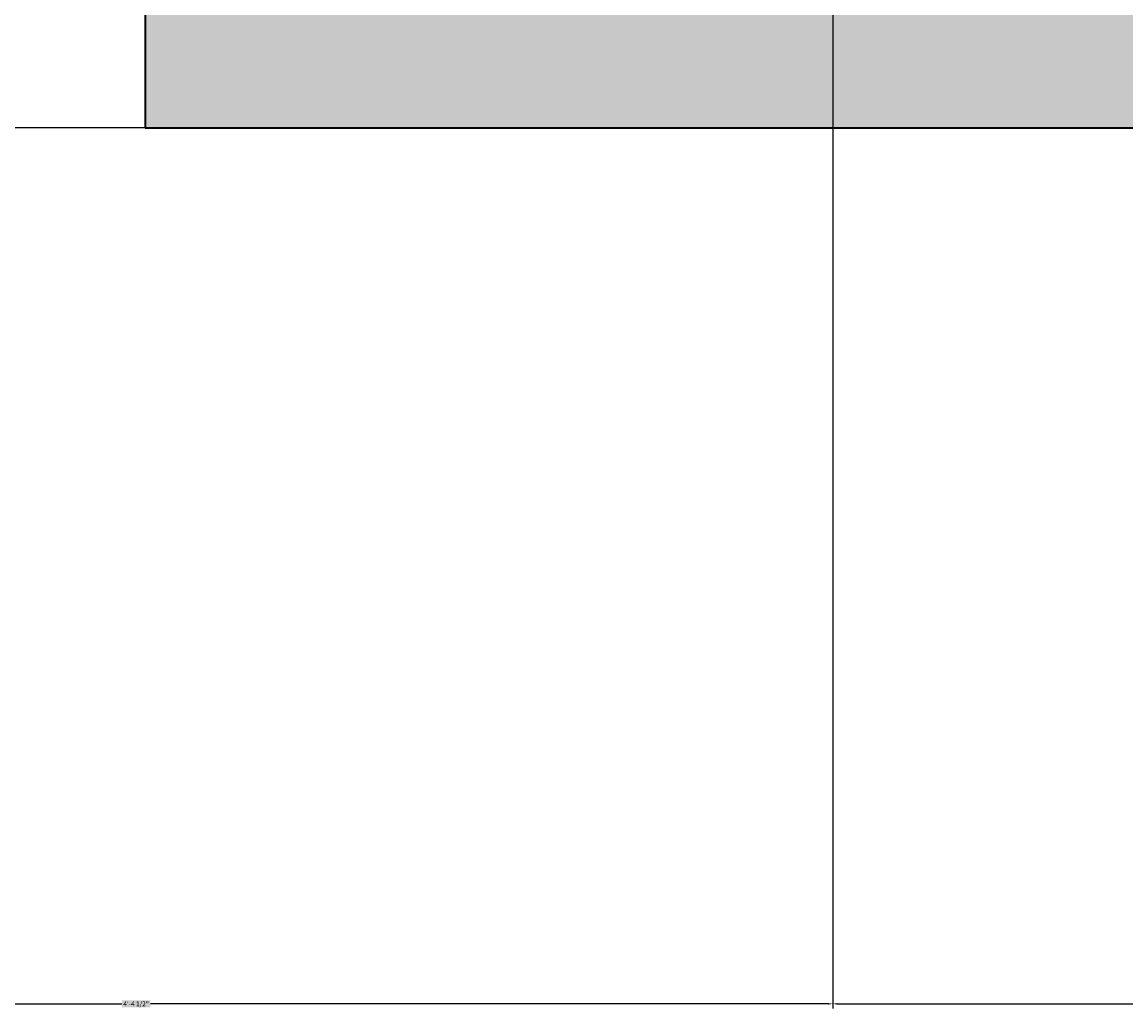
# Model space of a CAD drawing. Units: inches. Extents: x -301 to 715, y -607 to 364.
# Tile 2 of 141: x -66 to -24, y -574 to -536. Entities that reach past the tile are written whole.
import ezdxf

# ---------------------------------------------------------------- set-up
doc = ezdxf.new("R2010")
doc.units = ezdxf.units.IN
doc.header["$MEASUREMENT"] = 0
for name, color, linetype, lineweight in [('A-ANNO-DIMS', 2, 'Continuous', 18), ('A-SECT-PATT', 8, 'Continuous', 13), ('S-FNDN', 2, 'Continuous', 35)]:
    doc.layers.add(name, color=color, linetype=linetype, lineweight=lineweight)
doc.styles.get("Standard").update_dxf_attribs({"font": 'arial.ttf'})
doc.dimstyles.get("Standard").update_dxf_attribs({"dimtxt": 0.18, "dimasz": 0.18, "dimexe": 0.18, "dimexo": 0.0625, "dimgap": 0.09, "dimtad": 0, "dimtih": 1, "dimtoh": 1, "dimdec": 1, "dimzin": 0, "dimdsep": 46, "dimlunit": 4, "dimtxsty": 'Standard', "dimcen": 0.09, "dimclrd": 3, "dimclre": 4, "dimclrt": 6, "dimadec": 0, "dimazin": 0, "dimtfac": 1, "dimtdec": 1, "dimtofl": 0, "dimtmove": 0, "dimatfit": 3, "dimfxl": 1, "dimtfill": 2, "dimtfillclr": 51, "dimtolj": 1, "dimtzin": 0, "dimarcsym": 0})

# ---------------------------------------------------------------- blocks, each defined once
blk = doc.blocks.new('*D179')
at = {"layer": 'A-ANNO-DIMS', "color": 4, "lineweight": -2, "transparency": 16777216}
for p, q in [((-87.981, -433.54), (-87.981, -573.809)), ((-35.282, -463.54), (-35.282, -573.809))]:
    blk.add_line(p, q, dxfattribs=at)
at = {"layer": 'A-ANNO-DIMS', "color": 3, "lineweight": -2, "transparency": 16777216}
for p, q in [((-87.801, -573.629), (-62.174, -573.629)), ((-35.462, -573.629), (-61.089, -573.629))]:
    blk.add_line(p, q, dxfattribs=at)
at = {"layer": 'A-ANNO-DIMS', "color": 3, "transparency": 16777216}
for points in [[(-87.801, -573.599), (-87.801, -573.659), (-87.981, -573.629)], [(-35.462, -573.599), (-35.462, -573.659), (-35.282, -573.629)]]:
    blk.add_solid(points, dxfattribs=at)
at = {"layer": 'Defpoints', "color": 0, "transparency": 16777216}
for p in [(-87.981, -433.477), (-35.282, -463.477), (-35.282, -573.629)]:
    blk.add_point(p, dxfattribs=at)
at = {"layer": 'A-ANNO-DIMS', "color": 6, "transparency": 16777216, "insert": (-61.631, -573.629), "char_height": 0.18, "attachment_point": 5, "bg_fill": 1, "box_fill_scale": 1.25, "bg_fill_color": 51, "bg_fill_transparency": 0}
blk.add_mtext('\\A1;4\'-4 1/2"', dxfattribs=at)
blk = doc.blocks.new('*D180')
at = {"layer": 'A-ANNO-DIMS', "color": 4, "lineweight": -2, "transparency": 16777216}
for p, q in [((-35.282, -463.54), (-35.282, -573.809)), ((12.718, -463.54), (12.718, -573.809))]:
    blk.add_line(p, q, dxfattribs=at)
at = {"layer": 'A-ANNO-DIMS', "color": 3, "lineweight": -2, "transparency": 16777216}
for p, q in [((-35.102, -573.629), (-11.615, -573.629)), ((12.538, -573.629), (-10.949, -573.629))]:
    blk.add_line(p, q, dxfattribs=at)
at = {"layer": 'A-ANNO-DIMS', "color": 3, "transparency": 16777216}
for points in [[(-35.102, -573.599), (-35.102, -573.659), (-35.282, -573.629)], [(12.538, -573.599), (12.538, -573.659), (12.718, -573.629)]]:
    blk.add_solid(points, dxfattribs=at)
at = {"layer": 'Defpoints', "color": 0, "transparency": 16777216}
for p in [(-35.282, -463.477), (12.718, -463.477), (12.718, -573.629)]:
    blk.add_point(p, dxfattribs=at)
at = {"layer": 'A-ANNO-DIMS', "color": 6, "transparency": 16777216, "insert": (-11.282, -573.629), "char_height": 0.18, "attachment_point": 5, "bg_fill": 1, "box_fill_scale": 1.25, "bg_fill_color": 51, "bg_fill_transparency": 0}
blk.add_mtext('\\A1;4\'-0"', dxfattribs=at)
blk = doc.blocks.new('*D191')
at = {"layer": 'A-ANNO-DIMS', "color": 4, "lineweight": -2, "transparency": 16777216}
for p, q in [((129.193, -481.477), (-266.112, -481.477)), ((114.193, -540.477), (-266.112, -540.477))]:
    blk.add_line(p, q, dxfattribs=at)
at = {"layer": 'A-ANNO-DIMS', "color": 3, "lineweight": -2, "transparency": 16777216}
for p, q in [((-265.932, -481.657), (-265.932, -510.797)), ((-265.932, -540.297), (-265.932, -511.158))]:
    blk.add_line(p, q, dxfattribs=at)
at = {"layer": 'A-ANNO-DIMS', "color": 3, "transparency": 16777216}
for points in [[(-265.962, -481.657), (-265.902, -481.657), (-265.932, -481.477)], [(-265.962, -540.297), (-265.902, -540.297), (-265.932, -540.477)]]:
    blk.add_solid(points, dxfattribs=at)
at = {"layer": 'Defpoints', "color": 0, "transparency": 16777216}
for p in [(129.255, -481.477), (-265.932, -540.477), (114.255, -540.477)]:
    blk.add_point(p, dxfattribs=at)
at = {"layer": 'A-ANNO-DIMS', "color": 6, "transparency": 16777216, "insert": (-265.932, -510.977), "char_height": 0.18, "attachment_point": 5, "bg_fill": 1, "box_fill_scale": 1.25, "bg_fill_color": 51, "bg_fill_transparency": 0}
blk.add_mtext('\\A1;4\'-11"', dxfattribs=at)

msp = doc.modelspace()

# ---------------------------------------------------------------- hatches: boundary and pattern name
at = {"layer": 'A-SECT-PATT'}
h = msp.add_hatch(dxfattribs=at)
h.set_pattern_fill('AR-CONC', color=256, scale=0.5)
h.set_pattern_definition([(50, (10.3213, 33.8764), (3.586301, -0.31376), [0.375, -4.125]), (355, (10.3213, 33.8764), (-0.693757, 3.76096), [0.3, -3.3]), (100.45144, (10.62, 33.8502), (2.892544, 3.4472), [0.3187, -3.50571]), (46.1842, (10.3213, 34.8764), (5.336207, -0.827596), [0.5625, -6.1875]), (96.6356, (10.766, 34.8074), (4.67331, 4.870593), [0.47805, -5.25857]), (351.1842, (10.321, 34.8764), (4.67331, 4.870593), [0.45, -4.95]), (21, (10.8213, 34.6264), (2.984535, -2.013094), [0.375, -4.125]), (326, (10.8213, 34.6264), (1.216577, 3.62575), [0.3, -3.3]), (71.45144, (11.07, 34.4586), (4.201112, 1.612656), [0.3187, -3.50571]), (37.5, (10.3213, 33.8764), (0.0607993, 1.6644693), [0, -3.26, 0, -3.35, 0, -3.3125]), (7.5, (10.3213, 33.8764), (1.3153477, 1.9720586), [0, -1.91, 0, -3.185, 0, -1.2625]), (327.5, (9.2063, 33.8764), (2.6691122, -0.1127744), [0, -1.25, 0, -3.9, 0, -5.175]), (317.5, (8.7063, 33.8764), (2.915931, 0.500525), [0, -1.625, 0, -2.59, 0, -3.675])])
h.paths.add_polyline_path([(-56.282, -535.477), (-61.282, -535.477), (-61.282, -540.477), (-15.282, -540.477), (-15.282, -535.477), (-20.282, -535.477)])
h.paths.add_polyline_path([(119.255, -535.477), (114.255, -535.477), (114.255, -540.477), (163.255, -540.477), (163.255, -535.477), (158.255, -535.477)])
h.paths.add_polyline_path([(-206.282, -471.477), (-209.282, -471.477), (-209.282, -481.477), (-206.282, -481.477), (-194.282, -481.477), (-194.282, -471.477)])
h.paths.add_polyline_path([(-41.282, -481.477), (-41.282, -471.477), (-185.282, -471.477), (-185.282, -481.477), (-180.282, -481.477)])
h.paths.add_polyline_path([(134.255, -481.477), (134.255, -471.477), (-35.282, -471.477), (-35.282, -481.477), (-30.282, -481.477)])
h.paths.add_polyline_path([(155.218, -481.477), (158.218, -481.477), (158.218, -471.477), (153.218, -471.477), (143.218, -471.477), (143.218, -481.477), (148.255, -481.477)])
h.paths.add_polyline_path([(-193.88, -356.477), (-193.904, -361.477), (143.218, -361.477), (143.218, -356.477)])

# ---------------------------------------------------------------- linework, layer by layer
at = {"layer": 'S-FNDN'}
for p, q in [((-61.282, -535.477), (-61.282, -540.477)), ((-61.282, -540.477), (-15.282, -540.477))]:
    msp.add_line(p, q, dxfattribs=at)

# ---------------------------------------------------------------- dimensions: what is measured, and where the dimension line sits
at = {"layer": 'A-ANNO-DIMS'}
for base, p1, p2, picture, middle in [((-35.282, -573.629), (-87.981, -433.477), (-35.282, -463.477), '*D179', (-61.631, -573.629)), ((12.718, -573.629), (-35.282, -463.477), (12.718, -463.477), '*D180', (-11.282, -573.629))]:
    dim = msp.add_linear_dim(base=base, p1=p1, p2=p2, dimstyle='Standard', override={"dimdec": 1, "dimlfac": 1, "dimrnd": 0, "dimzin": 1, "dimdsep": 46, "dimlunit": 4, "dimfrac": 2}, dxfattribs=at)
    dim.commit()
    dim.dimension.update_dxf_attribs({"geometry": picture, "text_midpoint": middle})
dim = msp.add_linear_dim(base=(-265.932, -540.477), p1=(129.255, -481.477), p2=(114.255, -540.477), angle=90, dimstyle='Standard', override={"dimdec": 1, "dimlfac": 1, "dimrnd": 0, "dimzin": 1, "dimdsep": 46, "dimlunit": 4, "dimfrac": 2}, dxfattribs=at)
dim.commit()
dim.dimension.update_dxf_attribs({"geometry": '*D191', "text_midpoint": (-265.932, -510.977)})

doc.saveas('drawing.dxf')
